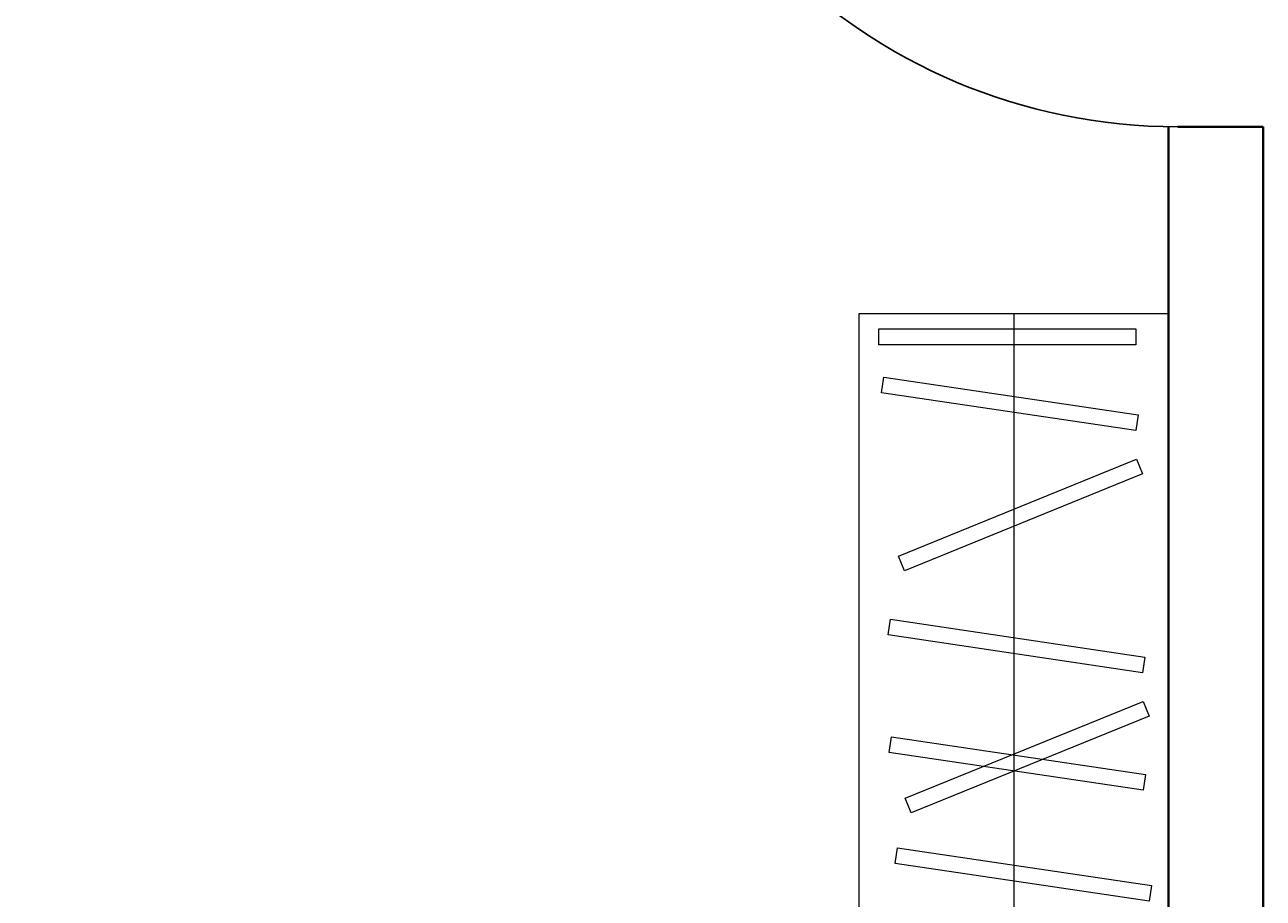
# Model space of a CAD drawing. Units: inches. Extents: x -46 to 1145, y -527 to 760.
# Tile 32 of 57: x 111 to 190, y 277 to 332. Entities that reach past the tile are written whole.
import ezdxf

# ---------------------------------------------------------------- set-up
doc = ezdxf.new("R2010")
doc.units = ezdxf.units.IN
doc.header["$MEASUREMENT"] = 0
for name, color, linetype, lineweight in [('A-ANNO-DIMS', 2, 'Continuous', 18), ('A-FLOR-CASE', 32, 'Continuous', 18), ('DOORS', 3, 'Continuous', 25), ('WALLS', 4, 'Continuous', 40)]:
    doc.layers.add(name, color=color, linetype=linetype, lineweight=lineweight)
doc.styles.get("Standard").update_dxf_attribs({"font": 'arial.ttf'})
doc.dimstyles.get("Standard").update_dxf_attribs({"dimtxt": 0.18, "dimasz": 0.18, "dimexe": 0.18, "dimexo": 0.0625, "dimgap": 0.09, "dimtad": 0, "dimtih": 1, "dimtoh": 1, "dimdec": 0, "dimzin": 0, "dimdsep": 46, "dimlunit": 3, "dimtxsty": 'Standard', "dimcen": 0.09, "dimadec": 0, "dimazin": 0, "dimtfac": 1, "dimtdec": 0, "dimtofl": 0, "dimtmove": 0, "dimatfit": 3, "dimfxl": 1, "dimtolj": 1, "dimtzin": 0, "dimarcsym": 0})

# ---------------------------------------------------------------- blocks, each defined once
blk = doc.blocks.new('*U2')
for p, q in [((0, 0), (0, -6)), ((40, 0), (40, -6))]:
    blk.add_line(p, q)
blk.add_lwpolyline([(0, 0), (0, 40), (1.75, 40), (1.75, 0)], close=True)
blk.add_arc((0, 0), 40, 0, 90)
blk = doc.blocks.new('WARDROBE')
blk.add_line((9.78, 0), (9.78, 83.246))
for points in [[(19.56, 0), (0, 0), (0, 83.246), (19.56, 83.246)], [(17.735, 78.486), (1.657, 80.876), (1.804, 81.869), (17.883, 79.479)], [(15.55, 76.351), (0.491, 70.229), (0.113, 71.159), (15.172, 77.281)], [(18.434, 71.396), (2.355, 73.786), (2.502, 74.779), (18.581, 72.389)], [(16.473, 65.03), (0.395, 67.42), (0.542, 68.413), (16.621, 66.023)], [(15.79, 61.003), (0.731, 54.88), (0.353, 55.81), (15.411, 61.933)], [(18.434, 57.618), (2.355, 60.008), (2.502, 61.001), (18.581, 58.611)], [(16.713, 49.682), (0.634, 52.071), (0.782, 53.064), (16.861, 50.674)], [(16.218, 45.124), (1.16, 39.002), (0.782, 39.931), (15.84, 46.054)], [(18.771, 41.016), (2.692, 43.406), (2.839, 44.399), (18.918, 42.009)], [(17.142, 33.803), (1.063, 36.193), (1.211, 37.186), (17.29, 34.796)], [(16.647, 30.67), (1.589, 24.548), (1.211, 25.477), (16.269, 31.6)], [(17.519, 26.78), (1.441, 29.169), (1.588, 30.162), (17.667, 27.772)], [(17.571, 19.349), (1.492, 21.739), (1.64, 22.732), (17.718, 20.342)], [(17.076, 15.353), (2.018, 9.231), (1.64, 10.161), (16.698, 16.283)], [(18, 4.032), (1.921, 6.422), (2.068, 7.415), (18.147, 5.025)], [(18.324, 0.979), (2.068, 0.979), (2.068, 1.983), (18.324, 1.983)]]:
    blk.add_lwpolyline(points, close=True)
blk = doc.blocks.new('*D685')
at = {"layer": 'A-ANNO-DIMS', "color": 0, "lineweight": -2, "transparency": 16777216}
for p, q in [((183.501, 700.889), (-46.216, 700.889)), ((-46.036, 700.709), (-46.036, 116.385)), ((-46.036, -468.302), (-46.036, 116.021)), ((12.501, -468.482), (-46.216, -468.482))]:
    blk.add_line(p, q, dxfattribs=at)
at = {"layer": 'A-ANNO-DIMS', "color": 0, "transparency": 16777216}
for points in [[(-46.066, 700.709), (-46.006, 700.709), (-46.036, 700.889)], [(-46.066, -468.302), (-46.006, -468.302), (-46.036, -468.482)]]:
    blk.add_solid(points, dxfattribs=at)
at = {"layer": 'Defpoints', "color": 0, "transparency": 16777216}
for p in [(-46.036, 700.889), (183.564, 700.889), (12.564, -468.482)]:
    blk.add_point(p, dxfattribs=at)
at = {"layer": 'A-ANNO-DIMS', "color": 0, "transparency": 16777216, "insert": (-46.036, 116.203), "char_height": 0.18, "attachment_point": 5}
blk.add_mtext('\\A1;1169.4', dxfattribs=at)

msp = doc.modelspace()

# ---------------------------------------------------------------- linework, layer by layer
at = {"layer": 'WALLS'}
for p, q in [((183.5637, 325.5663), (183.5637, 230.5176)), ((189.5637, 325.5613), (184.1637, 325.5613)), ((189.5637, 325.5613), (189.5637, 230.5176))]:
    msp.add_line(p, q, dxfattribs=at)

# ---------------------------------------------------------------- block references
at = {"layer": 'A-FLOR-CASE', "rotation": 180}
msp.add_blockref('WARDROBE', (183.5642, 313.7631), dxfattribs=at)
at = {"layer": 'DOORS', "xscale": -0.9, "yscale": 0.9, "zscale": 0.9, "rotation": 90}
msp.add_blockref('*U2', (184.1637, 361.5613), dxfattribs=at)

# ---------------------------------------------------------------- dimensions: what is measured, and where the dimension line sits
at = {"layer": 'A-ANNO-DIMS'}
dim = msp.add_linear_dim(base=(-46.0363, 700.8886), p1=(12.5637, -468.4824), p2=(183.5637, 700.8886), angle=90, dimstyle='Standard', override={"dimdec": 1, "dimlfac": 1, "dimrnd": 0, "dimzin": 0, "dimdsep": 46, "dimlunit": 2}, dxfattribs=at)
dim.commit()
dim.dimension.update_dxf_attribs({"geometry": '*D685', "text_midpoint": (-46.0363, 116.2031)})

doc.saveas('drawing.dxf')
